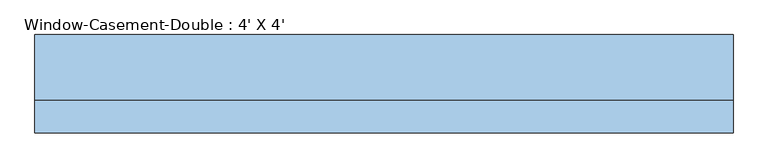
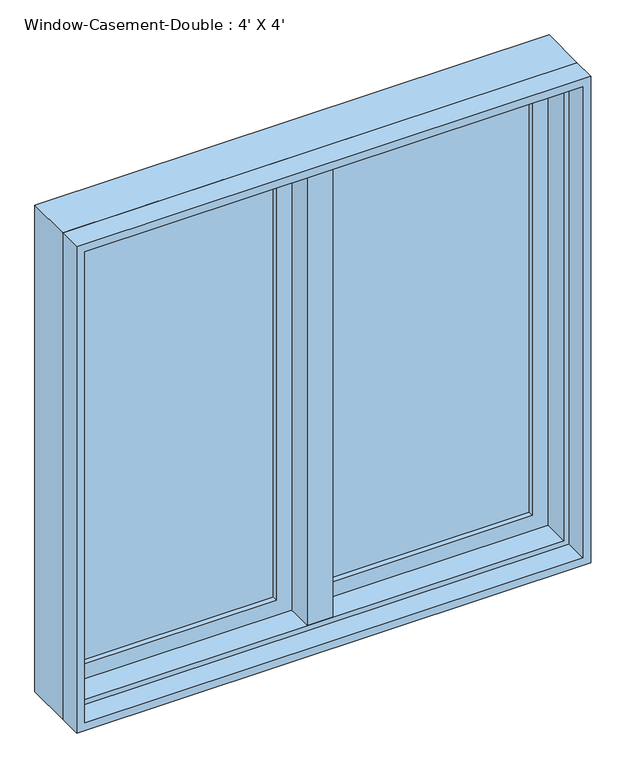
"""IFC4 building model written with IfcOpenShell, lengths in millimetres: window geometry, Window-Casement-Double : 4' X 4'."""

from ifc_helpers import new_model, si_unit, frame, origin, place, context, project, spatial, polyline, outline, extrude, faceted_brep, source, transform, mapped, element, save


def window_casement_double_4_x_4_83c2abfa(model_context):
    return source(origin(), model_context, "Body", "SolidModel", [
        faceted_brep([(577.85, 44.45, 2101.85), (577.85, -19.05, 2101.85), (-577.85, -19.05, 2101.85), (-577.85, 44.45, 2101.85), (596.9, 95.25, 2120.9), (596.9, 44.45, 2120.9), (-596.9, 44.45, 2120.9), (-596.9, 95.25, 2120.9), (609.6, -19.05, 2133.6), (609.6, 95.25, 2133.6), (-609.6, 95.25, 2133.6), (-609.6, -19.05, 2133.6), (-577.85, -19.05, 946.15), (-577.85, 44.45, 946.15), (-596.9, 44.45, 927.1), (-596.9, 95.25, 927.1), (-609.6, 95.25, 914.4), (-609.6, -19.05, 914.4), (577.85, -19.05, 946.15), (577.85, 44.45, 946.15), (596.9, 44.45, 927.1), (596.9, 95.25, 927.1), (609.6, 95.25, 914.4), (609.6, -19.05, 914.4)], [[[0, 1, 2, 3]], [[4, 5, 6, 7]], [[8, 9, 10, 11]], [[3, 2, 12, 13]], [[7, 6, 14, 15]], [[11, 10, 16, 17]], [[13, 12, 18, 19]], [[15, 14, 20, 21]], [[17, 16, 22, 23]], [[11, 17, 23, 8], [1, 18, 12, 2]], [[19, 18, 1, 0]], [[5, 20, 14, 6], [3, 13, 19, 0]], [[21, 20, 5, 4]], [[23, 22, 9, 8]], [[9, 22, 16, 10], [7, 15, 21, 4]]]),
        extrude(outline(polyline([(2133.6, -609.6), (914.4, -609.6), (914.4, 609.6), (2133.6, 609.6), (2133.6, -609.6)]), holes=[polyline([(2114.55, 590.55), (933.45, 590.55), (933.45, -590.55), (2114.55, -590.55), (2114.55, 590.55)])]), frame((0.0, -76.2, 0.0), z_axis=(0.0, 1.0, 0.0), x_axis=(0.0, 0.0, 1.0)), (0.0, 0.0, 1.0), 57.15),
        extrude(outline(polyline([(927.1, 596.9), (2120.9, 596.9), (2120.9, 9.525), (927.1, 9.525), (927.1, 596.9)]), holes=[polyline([(984.25, 66.675), (2063.75, 66.675), (2063.75, 539.75), (984.25, 539.75), (984.25, 66.675)])]), frame((0.0, 44.45, 0.0), z_axis=(0.0, 1.0, 0.0), x_axis=(0.0, 0.0, 1.0)), (0.0, 0.0, 1.0), 44.45),
        extrude(outline(polyline([(2120.9, -596.9), (927.1, -596.9), (927.1, -9.525), (2120.9, -9.525), (2120.9, -596.9)]), holes=[polyline([(2063.75, -66.675), (984.25, -66.675), (984.25, -539.75), (2063.75, -539.75), (2063.75, -66.675)])]), frame((0.0, 44.45, 0.0), z_axis=(0.0, 1.0, 0.0), x_axis=(0.0, 0.0, 1.0)), (0.0, 0.0, 1.0), 44.45),
        extrude(outline(polyline([(539.75, 76.2), (539.75, 69.85), (66.675, 69.85), (66.675, 76.2), (539.75, 76.2)])), frame((0.0, 0.0, 984.25), z_axis=(0.0, 0.0, 1.0), x_axis=(1.0, 0.0, 0.0)), (0.0, 0.0, 1.0), 1079.5),
        extrude(outline(polyline([(66.675, 57.15), (66.675, 63.5), (539.75, 63.5), (539.75, 57.15), (66.675, 57.15)])), frame((0.0, 0.0, 984.25), z_axis=(0.0, 0.0, 1.0), x_axis=(1.0, 0.0, 0.0)), (0.0, 0.0, 1.0), 1079.5),
        extrude(outline(polyline([(-66.675, 76.2), (-66.675, 69.85), (-539.75, 69.85), (-539.75, 76.2), (-66.675, 76.2)])), frame((0.0, 0.0, 984.25), z_axis=(0.0, 0.0, 1.0), x_axis=(1.0, 0.0, 0.0)), (0.0, 0.0, 1.0), 1079.5),
        extrude(outline(polyline([(-539.75, 57.15), (-539.75, 63.5), (-66.675, 63.5), (-66.675, 57.15), (-539.75, 57.15)])), frame((0.0, 0.0, 984.25), z_axis=(0.0, 0.0, 1.0), x_axis=(1.0, 0.0, 0.0)), (0.0, 0.0, 1.0), 1079.5),
        faceted_brep([(9.525, 95.25, 2120.9), (-9.525, 95.25, 2120.9), (-9.525, 44.45, 2120.9), (9.525, 44.45, 2120.9), (9.525, 95.25, 927.1), (9.525, 44.45, 927.1), (-9.525, 44.45, 927.1), (-9.525, 95.25, 927.1), (-9.525, 44.45, 946.15), (-9.525, 44.45, 2101.85), (-30.1625, 44.45, 946.15), (-30.1625, 44.45, 2101.85), (-30.1625, -19.05, 946.15), (-30.1625, -19.05, 2101.85), (30.1625, -19.05, 946.15), (30.1625, -19.05, 2101.85), (30.1625, 44.45, 946.15), (30.1625, 44.45, 2101.85), (9.525, 44.45, 946.15), (9.525, 44.45, 2101.85)], [[[0, 1, 2, 3]], [[4, 5, 6, 7]], [[1, 0, 4, 7]], [[2, 1, 7, 6, 8, 9]], [[9, 8, 10, 11]], [[11, 10, 12, 13]], [[13, 12, 14, 15]], [[15, 14, 16, 17]], [[17, 16, 18, 19]], [[0, 3, 19, 18, 5, 4]], [[18, 8, 6, 5]], [[9, 19, 3, 2]], [[8, 18, 16, 14, 12, 10]], [[19, 9, 11, 13, 15, 17]]]),
    ])


if __name__ == "__main__":
    model = new_model("IFC4")
    model_context = context("Model", 3, world=origin())
    ifc_project = project(units=[si_unit("LENGTHUNIT", "METRE", prefix="MILLI")], contexts=[model_context])
    site = spatial("IfcSite", under=ifc_project)
    building = spatial("IfcBuilding", under=site)
    placement = place(None, origin())
    window_casement_double_4_x_4_shape = window_casement_double_4_x_4_83c2abfa(model_context)
    element("IfcWindow", 1, ObjectType="Window-Casement-Double : 4' X 4'", at=placement, inside=building, context=model_context, shape_type="MappedRepresentation", body=[
        mapped(window_casement_double_4_x_4_shape, transform((0.0, 0.0, 0.0), x_axis=(1.0, 0.0, 0.0), y_axis=(0.0, 1.0, 0.0), z_axis=(0.0, 0.0, 1.0))),
    ])
    save(model, "model.ifc")

# Revit data of these elements
# Type "Window-Casement-Double : 4' X 4'"
#   Type Mark = "19"
#   Fire Rating = "0.5h"
#   Assembly Code = "B2020100"
#   Analytic Construction = "Double glazing - domestic"
#   Frame Extension [instance default] = 0' - 0 1/4"
#   Window Inset [instance default] = 0' - 0"
#   Wall Thickness [instance default] = 0' - 6"
#   Interior Wall Closure [instance default] = 0' - 2 1/4"
#   Half Width = 2' - 0"
#   Visual Light Transmittance = 0.81
#   Thermal Resistance (R) = 1.8146 (h·ft²·°F)/BTU
#   Solar Heat Gain Coefficient = 0.76
#   Rough Width = 4' - 0 1/2"
#   Rough Height = 4' - 0 1/2"
#   Height = 4' - 0"
#   Heat Transfer Coefficient (U) = 0.5511 BTU/(h·ft²·°F)
#   Exterior Wall Closure [instance default] = 0' - 1 1/4"
#   Extension Jamb [instance default] = 0' - 2 1/4"
#   Default Sill Height = 3' - 0"
#   Width = 4' - 0"
#   Muntin Visibility = yes
#   Interior Trim Visibility [instance default] = yes
#   Exterior Trim Visibility [instance default] = yes
#   Extension Jamb Visibility [instance default] = yes
#   Interior Trim Material = Wood - Stained
#   Muntin Pattern = Muntin Pattern_2x2 : Muntin Pattern_2x2
#   Interior Trim = Trim-Window-Interior-Flat : Picture Frame
#   Interior Frame Material = Wood - Stained
#   Glass Panel Material = Glass
#   Exterior Trim Material = Clad - White
#   Exterior Trim = Trim-Window-Exterior-Flat : with Sill
#   Exterior Frame Material = Clad - White
#   Wall Closure = (empty or 0)
# Element 1 (IfcWindow, "Window-Casement-Double : 4' X 4'")
#   Materials on its faces: "Wood - Stained", "Glass", "Clad - White"
# Materials
#   "Wood - Stained": class "Wood", colour RGB 224 178 126, transparency 0, Cost = 0
#   "Glass": class "Glass", colour RGB 0 128 192, transparency 0.75, Description = "Soda Lime Glass", Cost = 0
#   "Clad - White": class "Wood", colour RGB 242 242 238, transparency 0, Cost = 0
